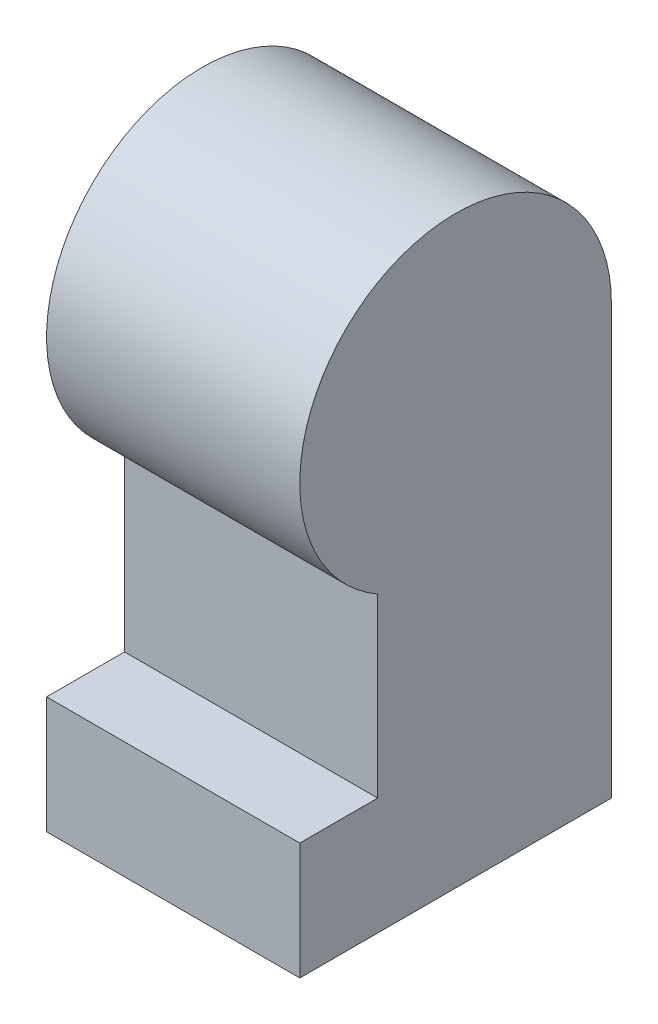
from build123d import *

# Parameters (mm, degrees)
LEG_BODY_DEPTH        = 3.25
LEG_SHELL_1MM_T       = -1
HIP_PIN_HOLE_3_REACH  = 15.388
HIP_PIN_HOLE_SKETCH_R = 1.5


with BuildPart() as part:
    # Leg Profile Sketch → Leg Body (new, symmetric)
    with BuildSketch(Plane(origin=(0, 0, 0), x_dir=(0, 0, -1), z_dir=(1, 0, 0))):
        with BuildLine():
            Line((4, 0), (4, -11))
            Line((4, -11), (-4, -11))
            Line((-4, -11), (-4, -8))
            Line((-4, -8), (-2, -8))
            Line((-2, -8), (-2, -3.464101615))
            ThreePointArc((-2, -3.464101615), (-2, 3.464101615), (4, 0))
        make_face()
    extrude(amount=LEG_BODY_DEPTH, both=True)

    # Leg Shell 1mm
    leg_shell_1mm_openings = [part.faces().sort_by_distance(p)[0] for p in [
        (0, -11, 0),
    ]]
    offset(amount=LEG_SHELL_1MM_T, openings=leg_shell_1mm_openings, kind=Kind.INTERSECTION)

    # Hip Pin Hole Sketch → Hip Pin Hole Ø3 (cut, up to next)
    with BuildSketch(Plane.ZY.offset(3.25), mode=Mode.PRIVATE) as hip_pin_hole_3_sk1:
        Circle(HIP_PIN_HOLE_SKETCH_R)
    hip_pin_hole_3_tool1 = extrude(hip_pin_hole_3_sk1.sketch, amount=-HIP_PIN_HOLE_3_REACH, mode=Mode.PRIVATE) & part.part
    add(hip_pin_hole_3_tool1.solids().sort_by_distance((-3.25, 0, 0))[0], mode=Mode.SUBTRACT)


solid = part.part
